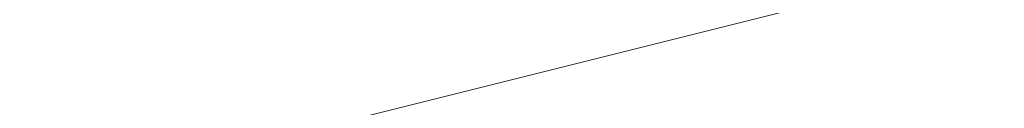
# Model space of a CAD drawing. Units: inches. Extents: x 2091 to 2899, y 967 to 2217.
# Tile 88 of 256: x 2251.2787 to 2251.29649, y 1099.9202 to 1099.92177. Entities that reach past the tile are written whole.
import ezdxf

# ---------------------------------------------------------------- set-up
doc = ezdxf.new("R2010")
doc.units = ezdxf.units.IN
doc.layers.add('A-ANNO-DIMS', color=2, linetype='Continuous', lineweight=18)
doc.layers.add('L-PLNT-TREE', color=94, linetype='Continuous', lineweight=13)
doc.layers.add('A-WALL-PATT', color=141, linetype='Continuous', lineweight=13, true_color=0xadddf7)
doc.styles.get("Standard").update_dxf_attribs({"font": 'arial.ttf'})
doc.dimstyles.new('ISO-25', dxfattribs={"dimtxt": 4, "dimasz": 4, "dimexe": 1.25, "dimexo": 0.625, "dimtad": 1, "dimdec": 0, "dimlunit": 3, "dimtxsty": 'Standard', "dimcen": 2.5, "dimadec": 0, "dimazin": 0, "dimtfac": 1, "dimtdec": 0, "dimtmove": 0, "dimatfit": 3, "dimfxl": 1, "dimarcsym": 0})

# ---------------------------------------------------------------- blocks, each defined once
blk = doc.blocks.new('*U29')
blk.add_line((-402.336, 12.192), (-451.104, 0))
blk = doc.blocks.new('*D71')
at = {"layer": 'A-ANNO-DIMS', "color": 0, "lineweight": -2, "transparency": 16777216}
for p, q in [((2212.143603, 1351.294059), (2212.143603, 969.464303)), ((2452.143603, 1351.294059), (2452.143603, 969.464303)), ((2216.143603, 970.714303), (2448.143603, 970.714303))]:
    blk.add_line(p, q, dxfattribs=at)
at = {"layer": 'A-ANNO-DIMS', "color": 0, "transparency": 16777216}
for points in [[(2216.143603, 971.38097), (2216.143603, 970.047636), (2212.143603, 970.714303)], [(2448.143603, 971.38097), (2448.143603, 970.047636), (2452.143603, 970.714303)]]:
    blk.add_solid(points, dxfattribs=at)
at = {"layer": 'Defpoints', "color": 0, "transparency": 16777216}
for p in [(2212.143603, 1351.919059), (2452.143603, 1351.919059), (2452.143603, 970.714303)]:
    blk.add_point(p, dxfattribs=at)
at = {"layer": 'A-ANNO-DIMS', "color": 0, "transparency": 16777216, "insert": (2332.143603, 973.381595), "char_height": 4, "attachment_point": 5}
blk.add_mtext('20\'-0"', dxfattribs=at)
blk = doc.blocks.new('*D75')
at = {"layer": 'A-ANNO-DIMS', "color": 0, "lineweight": -2, "transparency": 16777216}
for p, q in [((2212.143603, 1274.794059), (2212.143603, 969.464303)), ((2308.143603, 1274.794059), (2308.143603, 969.464303)), ((2216.143603, 970.714303), (2304.143603, 970.714303))]:
    blk.add_line(p, q, dxfattribs=at)
at = {"layer": 'A-ANNO-DIMS', "color": 0, "transparency": 16777216}
for points in [[(2216.143603, 971.38097), (2216.143603, 970.047636), (2212.143603, 970.714303)], [(2304.143603, 971.38097), (2304.143603, 970.047636), (2308.143603, 970.714303)]]:
    blk.add_solid(points, dxfattribs=at)
at = {"layer": 'Defpoints', "color": 0, "transparency": 16777216}
for p in [(2212.143603, 1275.419059), (2308.143603, 1275.419059), (2308.143603, 970.714303)]:
    blk.add_point(p, dxfattribs=at)
at = {"layer": 'A-ANNO-DIMS', "color": 0, "transparency": 16777216, "insert": (2260.143603, 973.381595), "char_height": 4, "attachment_point": 5}
blk.add_mtext('8\'-0"', dxfattribs=at)

msp = doc.modelspace()

# ---------------------------------------------------------------- hatches: boundary and pattern name
at = {"layer": 'A-WALL-PATT'}
h = msp.add_hatch(color=256, dxfattribs=at)
h.dxf.hatch_style = 1
h.paths.add_polyline_path([(2803.143603, 2050.919059), (2203.143603, 2050.919059), (2203.143603, 1090.919059), (2803.143603, 1090.919059)])
h.paths.add_polyline_path([(2635.79885, 1147.540465), (2674.524052, 1147.540465, 0.376086), (2678.529665, 1152.880202), (2678.529665, 1159.556473, 0.333335), (2674.524319, 1163.561846), (2674.524319, 1163.56185), (2674.524319, 1192.93439), (2635.805971, 1192.93439), (2597.087622, 1192.93439), (2597.087622, 1163.561846, 0.333335), (2593.082276, 1159.556473), (2593.082276, 1152.880202, 0.376086), (2597.087889, 1147.540465)], flags=0)
h.paths.add_polyline_path([(2436.010433, 1278.240778, 0.000483), (2435.952643, 1278.215027, -0.001328), (2435.935625, 1278.111693, -0.001711), (2436.11644, 1278.040758, 0.002185)], flags=0)
h.paths.add_polyline_path([(2794.143603, 1143.419059), (2794.143603, 1347.419059), (2543.370171, 1347.419059), (2543.370171, 1351.919059), (2794.143603, 1351.919059), (2794.143603, 1392.713555), (2793.947398, 1392.713555), (2793.947398, 1473.5369), (2794.143603, 1473.5369), (2794.143603, 1531.919059), (2650.143603, 1531.919059), (2650.143603, 1536.419059), (2794.143603, 1536.419059), (2794.143603, 1692.419059), (2609.375609, 1692.419059), (2609.375609, 1644.419059), (2604.875609, 1644.419059), (2604.875609, 1744.919059), (2609.375609, 1744.919059), (2609.375609, 1696.919059), (2794.143603, 1696.919059), (2794.143603, 1780.919059), (2609.643603, 1780.919059), (2493.875609, 1780.919059), (2493.875609, 1785.419059), (2609.643603, 1785.419059), (2794.143603, 1785.419059), (2794.143603, 1847.938821), (2793.951222, 1847.938821), (2793.951222, 1928.762166), (2794.143603, 1928.762166), (2794.143603, 1941.419059), (2614.143603, 1941.419059), (2614.143603, 1821.419059), (2609.643603, 1821.419059), (2609.643603, 1941.419059), (2392.143603, 1941.419059), (2392.143603, 1819.919059), (2387.643603, 1819.919059), (2387.643603, 1941.419059), (2212.143603, 1941.419059), (2212.143603, 1783.919059), (2392.143603, 1783.919059), (2392.143603, 1780.919059), (2212.143603, 1780.919059), (2212.143603, 1629.419059), (2387.643603, 1629.419059), (2387.643603, 1744.919059), (2392.143603, 1744.919059), (2392.143603, 1627.919059), (2317.143603, 1627.919059), (2317.143603, 1551.419059), (2317.143603, 1536.419059), (2459.383591, 1536.419059), (2459.383591, 1602.39648), (2463.883591, 1602.39648), (2463.883591, 1531.919059), (2456.643603, 1531.919059), (2456.643603, 1529.919059), (2452.143603, 1529.919059), (2452.143603, 1531.919059), (2312.643603, 1531.919059), (2312.643603, 1551.419059), (2306.143603, 1551.419059), (2306.143603, 1555.919059), (2308.143603, 1555.919059), (2308.143603, 1551.419059), (2312.643603, 1551.419059), (2312.643603, 1627.919059), (2212.143603, 1627.919059), (2212.143603, 1555.919059), (2270.143603, 1555.919059), (2270.143603, 1551.419059), (2212.143603, 1551.419059), (2212.143603, 1351.919059), (2272.143603, 1351.919059), (2272.143603, 1347.419059), (2212.143603, 1347.419059), (2212.143603, 1275.419059), (2308.143603, 1275.419059), (2308.143603, 1351.919059), (2452.143603, 1351.919059), (2452.143603, 1493.919059), (2456.643603, 1493.919059), (2456.643603, 1347.419059), (2312.643603, 1347.419059), (2312.643603, 1270.919059), (2212.143603, 1270.919059), (2212.143603, 1099.919059), (2281.237523, 1099.919059), (2282.871041, 1110.913803), (2282.008341, 1116.996603), (2278.557741, 1121.420403), (2268.205641, 1128.056203), (2272.087641, 1128.056203), (2273.812941, 1131.927003), (2279.420341, 1134.691903), (2285.027841, 1135.244903), (2287.615841, 1137.456803), (2288.047141, 1138.009803), (2289.341141, 1140.774703), (2291.066541, 1139.668703), (2292.360541, 1135.244903), (2295.379841, 1136.903803), (2296.242541, 1135.797903), (2297.105241, 1133.033003), (2300.124641, 1138.009803), (2303.143941, 1138.009803), (2304.437941, 1135.797903), (2303.143941, 1133.586003), (2306.594641, 1134.691903), (2307.888741, 1133.033003), (2310.908041, 1135.244903), (2313.927441, 1134.138903), (2315.62686, 1132.427102), (2308.320041, 1117.549603), (2290.203841, 1109.807903), (2288.909841, 1103.172103), (2289.272309, 1099.919059), (2434.918227, 1099.919059), (2431.593227, 1124.788059), (2429.930227, 1169.553059), (2430.927185, 1240.519694), (2435.658926, 1238.186126), (2437.135227, 1196.554059), (2438.798227, 1143.973059), (2442.678227, 1111.998059), (2446.558227, 1099.919059), (2794.143603, 1099.919059), (2794.143603, 1138.919059), (2548.032447, 1138.919059), (2548.032447, 1143.419059), (2548.032447, 1148.819059), (2546.668457, 1148.031559), (2528.685692, 1179.178622, 0.256256), (2512.032447, 1148.819059), (2512.032447, 1143.419059), (2512.032447, 1138.919059), (2507.532447, 1138.919059), (2507.532447, 1143.419059), (2507.532447, 1148.819059, 0.256256), (2490.879202, 1179.178622), (2472.896437, 1148.031559), (2471.532447, 1148.819059), (2471.532447, 1143.419059), (2467.032447, 1143.419059), (2467.032447, 1269.945786, 0.039061), (2460.909987, 1273.580059), (2467.032447, 1273.580059), (2467.032447, 1286.325364, 0.014511), (2465.216194, 1286.761905), (2467.032447, 1287.052576), (2467.032447, 1323.419059), (2471.532447, 1323.419059), (2471.532447, 1148.819059), (2489.532447, 1179.995973), (2490.896437, 1179.208473), (2490.879202, 1179.178622, -0.256256), (2507.532447, 1148.819059), (2507.532447, 1143.419059), (2512.032447, 1143.419059), (2512.032447, 1148.819059, -0.256256), (2528.685692, 1179.178622), (2528.668457, 1179.208473), (2530.032447, 1179.995973), (2548.032447, 1148.819059), (2548.032447, 1143.419059)], flags=16)
h.paths.add_polyline_path([(2607.768546, 1200.945083), (2607.768546, 1265.030625), (2597.087622, 1281.052011), (2619.784585, 1281.052011), (2627.795278, 1337.12686), (2635.79885, 1337.12686), (2643.816663, 1337.12686), (2651.827356, 1281.052011), (2674.524319, 1281.052011), (2663.843395, 1265.030625), (2663.843395, 1200.945083), (2635.805971, 1200.945083)], flags=0)
edge = h.paths.add_edge_path(flags=0)
edge.add_ellipse((13303.896215, 1272.998725), major_axis=(-10595.31304, 0.000001), ratio=0.842303870086, start_angle=0.6282372191, end_angle=0.6465540999, ccw=False)
edge.add_ellipse((2711.70045, 1156.852678), major_axis=(2.219769, 0), ratio=0.84230387, start_angle=111.535244, end_angle=180.628237, ccw=False)
edge.add_ellipse((13303.156292, 1272.998725), major_axis=(-10593.026306, 0), ratio=0.842303869544, start_angle=0.5282714718, end_angle=0.6465540971, ccw=False)
edge.add_line((2710.764596, 1175.333295), (2710.129986, 1175.333295))
edge.add_ellipse((2710.129986, 1176.579775), major_axis=(1.479846, 0), ratio=0.84230387, start_angle=180, end_angle=270, ccw=False)
edge.add_line((2708.65014, 1176.579775), (2708.65014, 1200.782914))
edge.add_ellipse((2710.129986, 1200.782914), major_axis=(1.479846, 0), ratio=0.84230387, start_angle=90, end_angle=180, ccw=False)
edge.add_line((2710.129986, 1202.029394), (2710.465075, 1202.029394))
edge.add_ellipse((13303.156292, 1272.998725), major_axis=(-10593.026306, 0), ratio=0.842303869544, start_angle=-0.0902290886, end_angle=0.3838667788, ccw=False)
edge.add_ellipse((2710.129986, 1290.927031), major_axis=(-1.479846, 0), ratio=0.84230387, start_angle=0, end_angle=90, ccw=False)
edge.add_line((2708.65014, 1290.927031), (2708.65014, 1315.13017))
edge.add_ellipse((2710.129986, 1315.13017), major_axis=(-1.479846, 0), ratio=0.84230387, start_angle=-90, end_angle=0, ccw=False)
edge.add_line((2710.129986, 1316.37665), (2710.706314, 1316.37665))
edge.add_ellipse((3238.40172, 1296.289566), major_axis=(528.234, 0), ratio=0.8423038695, start_angle=176.34957241, end_angle=177.82004969, ccw=False)
edge.add_ellipse((2775.063043, 1071.450696), major_axis=(313.307761, 0), ratio=0.8423038695, start_angle=102.12596555, end_angle=103.78052899, ccw=False)
edge.add_ellipse((2775.063043, 1078.305698), major_axis=(-305.302891, 0), ratio=0.8423038695, start_angle=-79.790461, end_angle=-77.55537271, ccw=False)
edge.add_ellipse((2695.141767, 1541.975383), major_axis=(-250.960216, 0), ratio=0.8423038695, start_angle=99.25656601, end_angle=102.55493264)
edge.add_line((2741.410326, 1334.214255), (2747.132545, 1337.378477))
edge.add_ellipse((2747.538616, 1336.857478), major_axis=(-0.739923, 0), ratio=0.8423039, start_angle=270, end_angle=307.93313, ccw=False)
edge.add_ellipse((2747.538616, 1336.857478), major_axis=(-0.739923, 0), ratio=0.8423039, start_angle=232.06687, end_angle=270, ccw=False)
edge.add_line((2747.944687, 1337.378477), (2753.666906, 1334.214255))
edge.add_ellipse((2799.935466, 1541.975383), major_axis=(250.960216, 0), ratio=0.8423038695, start_angle=257.44506736, end_angle=260.74343399)
edge.add_ellipse((2720.014189, 1078.305698), major_axis=(305.302891, 0), ratio=0.8423038695, start_angle=77.55537271, end_angle=79.790461, ccw=False)
edge.add_ellipse((2720.014189, 1071.450696), major_axis=(-313.307761, 0), ratio=0.8423038695, start_angle=256.21947101, end_angle=257.87403445, ccw=False)
edge.add_ellipse((2256.675512, 1296.289566), major_axis=(-528.234, 0), ratio=0.8423038695, start_angle=182.17995031, end_angle=183.65042759, ccw=False)
edge.add_line((2784.370918, 1316.37665), (2784.947247, 1316.37665))
edge.add_ellipse((2784.947247, 1315.13017), major_axis=(1.479846, 0), ratio=0.84230387, start_angle=0, end_angle=90, ccw=False)
edge.add_line((2786.427093, 1315.13017), (2786.427093, 1290.927031))
edge.add_ellipse((2784.947247, 1290.927031), major_axis=(1.479846, 0), ratio=0.84230387, start_angle=270, end_angle=360, ccw=False)
edge.add_ellipse((-7808.07906, 1272.998725), major_axis=(10593.026306, 0), ratio=0.842303869544, start_angle=-0.3838667788, end_angle=0.0902290886, ccw=False)
edge.add_line((2784.612157, 1202.029394), (2784.947247, 1202.029394))
edge.add_ellipse((2784.947247, 1200.782914), major_axis=(1.479846, 0), ratio=0.84230387, start_angle=0, end_angle=90, ccw=False)
edge.add_line((2786.427093, 1200.782914), (2786.427093, 1176.579775))
edge.add_ellipse((2784.947247, 1176.579775), major_axis=(-1.479846, 0), ratio=0.84230387, start_angle=90, end_angle=180, ccw=False)
edge.add_line((2784.947247, 1175.333295), (2784.312636, 1175.333295))
edge.add_ellipse((-7808.07906, 1272.998725), major_axis=(10593.026306, 0), ratio=0.842303869544, start_angle=-0.6186431963, end_angle=-0.5282714718, ccw=False)
edge.add_ellipse((2783.376783, 1156.852678), major_axis=(-2.219769, 0), ratio=0.84230387, start_angle=179.371763, end_angle=248.464757, ccw=False)
edge.add_ellipse((-7808.818983, 1272.998725), major_axis=(-10595.31304, 0.000004), ratio=0.842303865762, start_angle=179.3534459226, end_angle=179.3717628034, ccw=False)
edge.add_ellipse((2780.297303, 1153.500793), major_axis=(-5.246426, 0), ratio=0.84230387, start_angle=90, end_angle=179.353446, ccw=False)
edge.add_line((2780.297303, 1149.081708), (2714.77993, 1149.081708))
edge.add_ellipse((2714.77993, 1153.500793), major_axis=(5.246426, 0), ratio=0.84230387, start_angle=180.646554, end_angle=270, ccw=False)
edge = h.paths.add_edge_path(flags=0)
edge.add_line((2718.187367, 1151.007833), (2718.187367, 1170.472364))
edge.add_ellipse((2721.14706, 1170.472364), major_axis=(-2.959692, 0), ratio=0.84230387, start_angle=-90, end_angle=0, ccw=False)
edge.add_line((2721.14706, 1172.965324), (2773.930173, 1172.965324))
edge.add_ellipse((2773.930173, 1170.472364), major_axis=(-2.959692, 0), ratio=0.84230387, start_angle=180, end_angle=270, ccw=False)
edge.add_line((2776.889865, 1170.472364), (2776.889865, 1151.007833))
edge.add_line((2776.889865, 1151.007833), (2718.187367, 1151.007833))
edge = h.paths.add_edge_path(flags=0)
edge.add_line((2718.187367, 1180.23415), (2718.187367, 1199.057834))
edge.add_ellipse((2747.538616, 1320.39864), major_axis=(147.017924, 0), ratio=0.8423038695, start_angle=256.40186531, end_angle=283.59813469)
edge.add_line((2776.889865, 1199.057834), (2776.889865, 1180.23415))
edge.add_ellipse((2747.538616, 1301.574956), major_axis=(147.017924, 0), ratio=0.8423038695, start_angle=256.40186531, end_angle=283.59813469, ccw=False)
edge = h.paths.add_edge_path(flags=0)
edge.add_ellipse((13303.156292, 1272.998725), major_axis=(-10591.54646, 0), ratio=0.842303869555, start_angle=0.0555943135, end_angle=0.3777641939, ccw=False)
edge.add_line((2711.616859, 1262.72171), (2715.667408, 1249.495396))
edge.add_ellipse((6413.891963, 1241.691919), major_axis=(-3698.236159, 0), ratio=0.84230386955, start_angle=-0.120897369, end_angle=0.364076349)
edge.add_line((2715.761038, 1218.192455), (2711.934307, 1203.167361))
edge = h.paths.add_edge_path(flags=0)
edge.add_line((2718.187367, 1251.074566), (2716.002485, 1267.450435))
edge.add_ellipse((2742.151175, 1202.18954), major_axis=(81.772585, 0), ratio=0.84230387, start_angle=94.27742096, end_angle=111.8349538, ccw=False)
edge.add_line((2737.009748, 1270.930626), (2758.067484, 1270.930626))
edge.add_ellipse((2752.926058, 1202.18954), major_axis=(81.772585, 0), ratio=0.84230387, start_angle=68.1650462, end_angle=85.72257904, ccw=False)
edge.add_line((2779.074747, 1267.450435), (2776.889865, 1251.074566))
edge.add_ellipse((2750.338059, 1187.885356), major_axis=(79.579664, 0), ratio=0.84230387, start_angle=67.20808512, end_angle=85.1299304)
edge.add_line((2756.034656, 1254.743656), (2739.042576, 1254.743656))
edge.add_ellipse((2744.739174, 1187.885356), major_axis=(79.579664, 0), ratio=0.84230387, start_angle=94.8700696, end_angle=112.79191488)
edge = h.paths.add_edge_path(flags=0)
edge.add_line((2783.142926, 1203.167361), (2779.316194, 1218.192455))
edge.add_ellipse((-918.81473, 1241.691919), major_axis=(3698.236159, 0), ratio=0.84230386955, start_angle=-0.364076349, end_angle=0.120897369)
edge.add_line((2779.409825, 1249.495396), (2783.460373, 1262.72171))
edge.add_ellipse((-7808.07906, 1272.998725), major_axis=(-10591.54646, 0), ratio=0.84230386954, start_angle=179.6222358061, end_angle=179.9444056865, ccw=False)
edge = h.paths.add_edge_path(flags=0)
edge.add_ellipse((2734.200892, 1286.69044), major_axis=(-0.356609, 6.340078), ratio=0.60383358, start_angle=89.0020143, end_angle=253.657408, ccw=False)
edge.add_line((2730.369001, 1286.541806), (2730.369001, 1301.35198))
edge.add_line((2730.369001, 1301.35198), (2735.913311, 1305.214803))
edge.add_ellipse((2736.384917, 1304.734561), major_axis=(0.739923, 0), ratio=0.8423039, start_angle=90, end_angle=134.480211, ccw=False)
edge.add_line((2736.384917, 1305.357801), (2738.032783, 1305.357801))
edge.add_line((2738.032783, 1305.357801), (2738.032783, 1307.707927))
edge.add_ellipse((2794.201642, 1307.707927), major_axis=(56.168859, 0), ratio=0.84230387, start_angle=150.5614304, end_angle=180, ccw=False)
edge.add_ellipse((2700.875591, 1307.707927), major_axis=(-56.168859, 0), ratio=0.84230387, start_angle=180, end_angle=209.4385696, ccw=False)
edge.add_line((2757.04445, 1307.707927), (2757.04445, 1305.357801))
edge.add_line((2757.04445, 1305.357801), (2758.692316, 1305.357801))
edge.add_ellipse((2758.692316, 1304.734561), major_axis=(-0.739923, 0), ratio=0.8423039, start_angle=225.519789, end_angle=270, ccw=False)
edge.add_line((2759.163922, 1305.214803), (2764.708231, 1301.35198))
edge.add_line((2764.708231, 1301.35198), (2764.708231, 1286.541806))
edge.add_ellipse((2760.87634, 1286.69044), major_axis=(0.356609, 6.340078), ratio=0.60383358, start_angle=106.342592, end_angle=270.9979857, ccw=False)
edge.add_line((2757.04445, 1285.79709), (2757.04445, 1307.707927))
edge.add_ellipse((2700.875591, 1307.707927), major_axis=(-56.168859, 0), ratio=0.84230387, start_angle=180, end_angle=209.4385696)
edge.add_ellipse((2794.201642, 1307.707927), major_axis=(56.168859, 0), ratio=0.84230387, start_angle=150.5614304, end_angle=180)
edge.add_line((2738.032783, 1307.707927), (2738.032783, 1285.79709))
h.paths.add_polyline_path([(2417.812273, 1104.449704), (2413.492273, 1102.529704), (2410.612273, 1103.969704), (2409.172273, 1106.369704), (2407.252273, 1107.329704), (2406.292273, 1109.729704), (2405.332273, 1114.049704), (2405.332273, 1117.889704), (2406.292273, 1120.129704), (2407.252273, 1119.809704), (2408.848322, 1118.327658), (2410.173945, 1119.42417), (2410.211273, 1120.405704), (2411.040731, 1121.419054), (2410.699273, 1119.858704), (2410.173945, 1119.42417), (2410.088452, 1117.176109), (2411.132836, 1116.206324), (2413.972273, 1119.329704), (2416.852273, 1120.769704), (2416.869721, 1120.798784), (2417.035071, 1119.405116), (2417.896213, 1118.143384), (2418.292273, 1118.369704), (2419.544447, 1120.039269), (2419.360915, 1118.387487), (2419.032108, 1119.356151), (2418.398939, 1118.511926), (2419.252273, 1114.529704), (2418.794091, 1107.198795)], flags=0)
h.paths.add_polyline_path([(2508.870171, 1347.419059), (2508.370171, 1347.419059), (2508.370171, 1351.919059), (2508.870171, 1351.919059)], flags=0)
h.paths.add_polyline_path([(2473.370171, 1347.419059), (2472.370171, 1347.419059), (2467.870171, 1347.419059), (2467.870171, 1455.419059), (2472.370171, 1455.419059), (2472.370171, 1352.419059), (2473.370171, 1352.419059)], flags=0)
h.paths.add_polyline_path([(2352.106244, 1217.446197), (2349.226244, 1218.886197), (2347.786244, 1221.286197), (2345.866244, 1222.246197), (2344.906244, 1224.646197), (2343.946244, 1228.966197), (2343.946244, 1232.806197), (2344.906244, 1235.046197), (2345.866244, 1234.726197), (2347.462293, 1233.244152), (2348.787916, 1234.340663), (2348.825244, 1235.322197), (2349.654702, 1236.335547), (2349.313244, 1234.775197), (2348.787916, 1234.340663), (2348.702423, 1232.092603), (2349.746807, 1231.122817), (2352.586244, 1234.246197), (2355.466244, 1235.686197), (2355.483692, 1235.715277), (2355.649043, 1234.321609), (2356.510185, 1233.059877), (2356.906244, 1233.286197), (2358.158418, 1234.955762), (2357.974887, 1233.30398), (2357.646079, 1234.272644), (2357.012911, 1233.428419), (2357.866244, 1229.446197), (2357.408062, 1222.115288), (2356.426244, 1219.366197)], flags=0)
h.paths.add_polyline_path([(2348.2968, 1112.22442), (2347.0138, 1112.31042), (2345.5298, 1114.12742), (2345.7318, 1115.85842), (2346.8118, 1116.98242), (2346.8118, 1114.64642), (2345.8668, 1114.21442), (2346.8798, 1114.30042)], flags=0)
h.paths.add_polyline_path([(2347.0138, 1110.92642), (2346.2718, 1110.49342), (2346.6098, 1111.18642)], flags=0)
h.paths.add_polyline_path([(2345.8668, 1118.19442), (2345.5298, 1117.32942), (2343.7078, 1118.02142), (2344.3828, 1118.62642)], flags=0)
h.paths.add_polyline_path([(2346.6768, 1109.28242), (2346.0698, 1108.07142), (2345.8668, 1110.06142)], flags=0)
h.paths.add_polyline_path([(2345.0568, 1119.75142), (2343.6398, 1119.75142), (2343.9778, 1121.13542)], flags=0)
h.paths.add_polyline_path([(2345.2598, 1116.55042), (2345.1248, 1115.85842), (2344.9218, 1115.68542), (2344.7198, 1116.37742)], flags=0)
h.paths.add_polyline_path([(2345.6648, 1112.31042), (2345.4618, 1111.53242), (2344.0448, 1111.96442), (2344.6518, 1112.57042)], flags=0)
h.paths.add_polyline_path([(2345.1918, 1113.34942), (2344.4498, 1113.86842), (2344.7198, 1114.38742)], flags=0)
h.paths.add_polyline_path([(2344.6518, 1116.80942), (2344.1798, 1115.68542), (2344.6518, 1115.33942), (2343.9098, 1114.90642), (2343.0328, 1115.94442), (2343.6398, 1116.46342)], flags=0)
h.paths.add_polyline_path([(2345.8668, 1106.68642), (2344.9898, 1105.56242), (2344.5168, 1106.60042)], flags=0)
h.paths.add_polyline_path([(2344.8548, 1110.06142), (2344.5168, 1109.28242), (2344.1128, 1109.71542)], flags=0)
h.paths.add_polyline_path([(2344.0448, 1113.52242), (2343.4378, 1113.08942), (2342.7628, 1113.95442)], flags=0)
h.paths.add_polyline_path([(2344.3148, 1111.01242), (2342.9648, 1110.32042), (2342.9648, 1111.09942)], flags=0)
h.paths.add_polyline_path([(2345.1248, 1104.69742), (2344.5848, 1103.74542), (2344.4498, 1104.26442)], flags=0)
h.paths.add_polyline_path([(2342.8298, 1121.22242), (2341.7498, 1120.53042), (2340.5358, 1121.04942), (2340.1308, 1121.82842), (2340.6708, 1122.95242), (2341.1428, 1121.82842), (2341.6148, 1122.00142)], flags=0)
h.paths.add_polyline_path([(2342.9648, 1119.75142), (2343.0328, 1118.45342), (2342.0878, 1118.02142), (2342.0198, 1119.49142)], flags=0)
h.paths.add_polyline_path([(2342.6948, 1116.89642), (2341.9528, 1116.63642), (2342.0198, 1117.32942)], flags=0)
h.paths.add_polyline_path([(2343.0328, 1112.22442), (2342.0198, 1111.79142), (2341.5478, 1112.22442), (2342.3578, 1113.34942)], flags=0)
h.paths.add_polyline_path([(2343.7748, 1104.43742), (2342.6278, 1102.88042), (2342.6948, 1104.61042), (2343.4378, 1105.12942)], flags=0)
h.paths.add_polyline_path([(2342.0198, 1115.07942), (2340.8058, 1115.51242), (2340.9408, 1116.37742)], flags=0)
h.paths.add_polyline_path([(2341.4808, 1120.09742), (2341.4808, 1119.40542), (2341.0758, 1119.57842), (2341.1428, 1120.09742)], flags=0)
h.paths.add_polyline_path([(2341.8178, 1114.47342), (2340.9408, 1113.08942), (2340.8058, 1114.56042)], flags=0)
h.paths.add_polyline_path([(2341.1428, 1118.54042), (2340.9408, 1116.98242), (2339.0508, 1117.67542), (2339.0508, 1118.62642)], flags=0)
h.paths.add_polyline_path([(2342.6948, 1101.66842), (2341.9528, 1101.84142), (2342.5598, 1102.36142)], flags=0)
h.paths.add_polyline_path([(2340.3328, 1119.66542), (2338.4438, 1119.57842), (2337.9038, 1120.35742), (2339.6578, 1120.61642)], flags=0)
h.paths.add_polyline_path([(2340.3328, 1115.33942), (2340.0628, 1113.69542), (2339.3878, 1115.33942)], flags=0)
h.paths.add_polyline_path([(2341.8178, 1103.83142), (2341.5478, 1102.88042), (2341.1428, 1103.65842)], flags=0)
h.paths.add_polyline_path([(2339.0508, 1122.86642), (2337.2958, 1121.82842), (2337.0938, 1123.12542), (2337.7688, 1123.81842)], flags=0)
h.paths.add_polyline_path([(2339.1178, 1121.74142), (2338.8478, 1121.22242), (2338.1738, 1121.04942), (2338.3758, 1121.56842)], flags=0)
h.paths.add_polyline_path([(2339.1858, 1119.31942), (2338.6458, 1118.71342), (2338.2408, 1118.10742), (2338.2408, 1118.88642)], flags=0)
h.paths.add_polyline_path([(2341.1428, 1101.92842), (2340.6028, 1101.23642), (2340.0628, 1101.84142), (2340.6028, 1102.36142)], flags=0)
h.paths.add_polyline_path([(2337.6338, 1117.76142), (2336.6208, 1118.28042), (2337.2958, 1118.97242)], flags=0)
h.paths.add_polyline_path([(2336.8238, 1119.57842), (2334.7988, 1118.97242), (2335.2038, 1120.35742), (2336.5538, 1120.87642)], flags=0)
h.paths.add_polyline_path([(2339.1178, 1100.45742), (2337.3638, 1100.54342), (2336.7558, 1101.23642)], flags=0)
h.paths.add_polyline_path([(2336.3508, 1122.43342), (2336.0138, 1121.91442), (2334.9338, 1122.43342), (2334.5288, 1123.47142), (2335.7438, 1122.77942)], flags=0)
h.paths.add_polyline_path([(2334.7318, 1120.87642), (2334.2588, 1120.35742), (2334.0568, 1120.78942), (2334.5968, 1121.30842)], flags=0)
h.paths.add_polyline_path([(2334.4618, 1122.17442), (2332.5718, 1121.30842), (2331.3568, 1122.17442), (2332.0998, 1122.86642)], flags=0)
h.paths.add_polyline_path([(2334.2588, 1118.54042), (2333.3818, 1118.45342), (2333.6518, 1119.31942)], flags=0)
h.paths.add_polyline_path([(2335.5418, 1102.27442), (2334.1918, 1102.62042), (2335.2718, 1103.31242)], flags=0)
h.paths.add_polyline_path([(2332.7068, 1119.66542), (2331.6948, 1120.44342), (2332.5048, 1120.78942)], flags=0)
h.paths.add_polyline_path([(2334.7318, 1101.14942), (2333.5168, 1101.58242), (2333.9888, 1101.75542)], flags=0)
h.paths.add_polyline_path([(2332.6398, 1116.63642), (2331.0868, 1116.29042), (2331.9648, 1118.19442)], flags=0)
h.paths.add_polyline_path([(2330.7498, 1121.56842), (2330.2768, 1120.27042), (2328.5228, 1119.31942), (2328.9948, 1121.04942)], flags=0)
h.paths.add_polyline_path([(2330.7498, 1118.62642), (2330.0078, 1117.50242), (2329.8728, 1118.02142)], flags=0)
h.paths.add_polyline_path([(2332.0998, 1102.36142), (2330.5468, 1102.01442), (2331.6948, 1102.96642)], flags=0)
h.paths.add_polyline_path([(2329.5348, 1113.60842), (2329.0628, 1112.31042), (2328.5898, 1113.34942)], flags=0)
h.paths.add_polyline_path([(2328.3878, 1117.84842), (2327.5098, 1116.55042), (2327.1728, 1117.76142)], flags=0)
h.paths.add_polyline_path([(2329.7378, 1106.51342), (2329.5348, 1105.30242), (2328.2528, 1106.08142)], flags=0)
h.paths.add_polyline_path([(2328.6578, 1114.38742), (2328.0498, 1114.12742), (2328.3198, 1114.90642)], flags=0)
h.paths.add_polyline_path([(2328.3198, 1112.22442), (2327.1058, 1112.13742), (2326.7008, 1112.65642)], flags=0)
h.paths.add_polyline_path([(2326.9028, 1115.25242), (2326.7008, 1114.12742), (2325.2158, 1113.60842), (2326.0928, 1115.33942)], flags=0)
h.paths.add_polyline_path([(2326.6328, 1108.33042), (2326.0928, 1107.37942), (2325.8908, 1108.50342), (2326.4978, 1109.10942)], flags=0)
h.paths.add_polyline_path([(2615.143603, 1531.919059), (2609.643603, 1531.919059), (2609.643603, 1620.419059), (2614.143603, 1620.419059), (2614.143603, 1536.419059), (2615.143603, 1536.419059)], flags=0)
h.paths.add_polyline_path([(2545.143603, 1563.419059), (2464.143603, 1563.419059), (2464.143603, 1632.419059), (2509.143603, 1632.419059), (2509.143603, 1627.919059), (2509.143603, 1603.919059), (2468.643603, 1603.919059), (2468.643603, 1567.919059), (2540.643603, 1567.919059), (2540.643603, 1591.919059), (2545.143603, 1591.919059)], flags=0)
h.paths.add_polyline_path([(2388.969048, 1549.985735), (2357.434181, 1549.985735), (2357.434181, 1623.360778), (2399.362777, 1623.360778), (2435.689465, 1623.360778), (2435.592547, 1602.559273), (2435.592547, 1602.39648), (2388.969048, 1602.39648)], flags=0)
h.paths.add_polyline_path([(2388.880628, 1555.809151), (2374.904429, 1555.809151), (2374.904429, 1600.571564), (2374.904429, 1615.457645), (2406.350877, 1615.457645), (2406.350877, 1618.939431), (2412.174293, 1615.457645), (2406.350877, 1611.97586), (2406.350877, 1615.457645), (2388.880628, 1615.457645)], flags=0)
h.paths.add_polyline_path([(2568.875609, 1644.419059), (2453.375609, 1644.419059), (2453.375609, 1785.419059), (2457.875609, 1785.419059), (2457.875609, 1648.919059), (2568.875609, 1648.919059)], flags=0)
h.paths.add_polyline_path([(2212.143603, 1945.919059), (2212.143603, 2041.919059), (2794.143603, 2041.919059), (2794.143603, 1945.919059)], flags=16)
h.paths.add_polyline_path([(2271.082728, 1964.317238), (2776.852968, 1964.317238), (2776.852968, 2037.169623), (2271.082728, 2037.169623)], flags=8)
h.paths.add_polyline_path([(2380.649285, 1536.824144), (2461.040809, 1536.824144), (2461.040809, 1554.652587), (2380.649285, 1554.652587)], flags=8)
h.paths.add_polyline_path([(2240.755709, 1609.725451), (2309.185829, 1609.725451), (2309.185829, 1617.698204), (2240.755709, 1617.698204)], flags=8)
h.paths.add_polyline_path([(2212.677255, 1313.504102), (2282.59152, 1313.504102), (2282.59152, 1322.745239), (2212.677255, 1322.745239)], flags=8)
h.paths.add_polyline_path([(2457.111976, 1114.778574), (2558.481581, 1114.778574), (2558.481581, 1142.219682), (2457.111976, 1142.219682)], flags=8)
h.paths.add_polyline_path([(2473.442337, 1273.010067), (2604.641226, 1273.010067), (2604.641226, 1318.346935), (2473.442337, 1318.346935)], flags=8)
h.paths.add_polyline_path([(2638.876302, 1626.977432), (2684.250367, 1627.976738), (2684.038483, 1637.597494), (2638.664417, 1636.598188)], flags=8)
h.paths.add_polyline_path([(2537.590554, 1453.793447), (2628.389547, 1453.793447), (2628.389547, 1475.344811), (2537.590554, 1475.344811)], flags=8)
h.paths.add_polyline_path([(2504.137638, 1714.632397), (2554.647187, 1714.632397), (2554.647187, 1730.237712), (2504.137638, 1730.237712)], flags=8)
h.paths.add_polyline_path([(2487.501181, 1575.651872), (2535.097121, 1575.651872), (2535.097121, 1598.377646), (2487.501181, 1598.377646)], flags=8)
h.paths.add_polyline_path([(2709.0994, 1735.710278), (2740.016601, 1735.710278), (2740.016601, 1749.937641), (2709.0994, 1749.937641)], flags=8)
h.paths.add_polyline_path([(2442.438424, 1792.171657), (2564.728835, 1792.171657), (2564.728835, 1842.000163), (2442.438424, 1842.000163)], flags=8)
h.paths.add_polyline_path([(2655.815801, 1809.644076), (2789.520142, 1806.693796), (2790.084977, 1832.291638), (2656.380635, 1835.241918)], flags=8)
h.paths.add_polyline_path([(2234.842697, 1797.720143), (2368.592851, 1794.768852), (2369.160718, 1820.504132), (2235.410564, 1823.455423)], flags=8)
h.paths.add_polyline_path([(2245.138466, 1644.006335), (2398.427733, 1640.6239), (2398.994842, 1666.32482), (2245.705575, 1669.707255)], flags=8)
h.paths.add_polyline_path([(2306.142847, 1431.168519), (2413.768314, 1428.793687), (2414.333148, 1454.391529), (2306.707682, 1456.76636)], flags=8)
h.paths.add_polyline_path([(2306.834582, 1458.233145), (2393.380484, 1456.323449), (2393.932808, 1481.354358), (2307.386907, 1483.264054)], flags=8)

# ---------------------------------------------------------------- block references
at = {"layer": 'L-PLNT-TREE', "xscale": 0.0393700787401575, "yscale": 0.0393700787401575, "zscale": 0.0393700787401575}
msp.add_blockref('*U29', (2269.041014, 1099.919059), dxfattribs=at)

# ---------------------------------------------------------------- dimensions: what is measured, and where the dimension line sits
at = {"layer": 'A-ANNO-DIMS'}
for base, p1, p2, picture, middle in [((2452.143603, 970.714303), (2212.143603, 1351.919059), (2452.143603, 1351.919059), '*D71', (2332.143603, 973.381595)), ((2308.143603, 970.714303), (2212.143603, 1275.419059), (2308.143603, 1275.419059), '*D75', (2260.143603, 973.381595))]:
    dim = msp.add_linear_dim(base=base, p1=p1, p2=p2, dimstyle='ISO-25', override={"dimdec": 1, "dimlfac": 1, "dimrnd": 0, "dimzin": 1, "dimdsep": 46, "dimlunit": 4, "dimfrac": 2}, dxfattribs=at)
    dim.commit()
    dim.dimension.update_dxf_attribs({"geometry": picture, "text_midpoint": middle})

doc.saveas('drawing.dxf')
